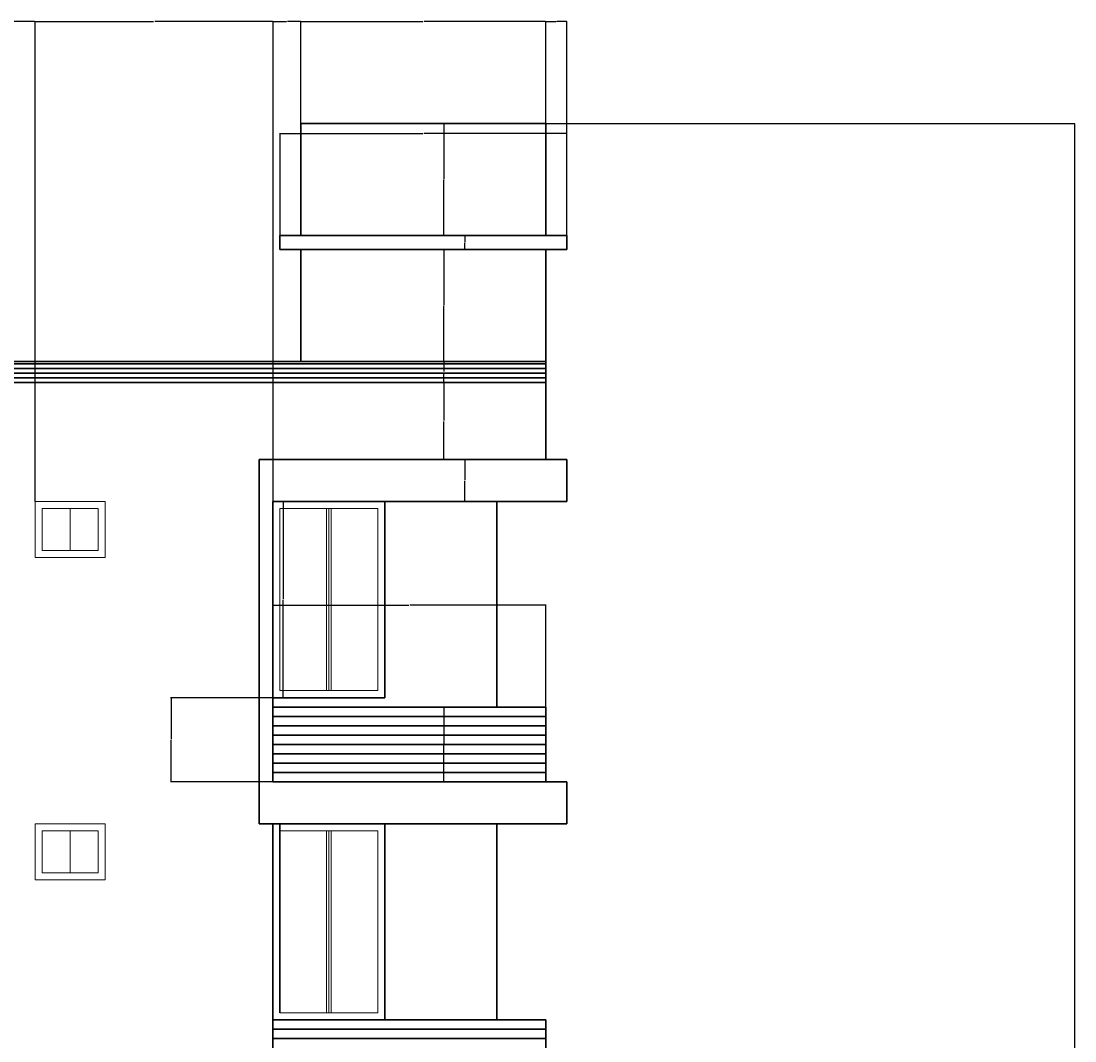
# Model space of a CAD drawing. Units: inches. Extents: x 2136 to 3058, y 322 to 1274.
# Tile 3 of 3: x 2606 to 3058, y 837 to 1274. Entities that reach past the tile are written whole.
import ezdxf

# ---------------------------------------------------------------- set-up
doc = ezdxf.new("R2010")
doc.units = ezdxf.units.IN
for name, color, linetype, lineweight in [('A-ANNO-DIMS', 2, 'Continuous', 18), ('A-ELEV', 7, 'Continuous', 35), ('A-GLAZ', 4, 'Continuous', 18)]:
    doc.layers.add(name, color=color, linetype=linetype, lineweight=lineweight)
doc.styles.get("Standard").update_dxf_attribs({"font": 'arial.ttf'})
doc.dimstyles.get("Standard").update_dxf_attribs({"dimtxt": 0.18, "dimasz": 0.18, "dimexe": 0.18, "dimexo": 0.0625, "dimgap": 0.09, "dimtad": 0, "dimtih": 1, "dimtoh": 1, "dimdec": 4, "dimzin": 0, "dimdsep": 46, "dimtxsty": 'Standard', "dimcen": 0.09, "dimadec": 0, "dimazin": 0, "dimtfac": 1, "dimtdec": 4, "dimtofl": 0, "dimtmove": 0, "dimatfit": 3, "dimfxl": 1, "dimtolj": 1, "dimtzin": 0, "dimarcsym": 0})

# ---------------------------------------------------------------- blocks, each defined once
blk = doc.blocks.new('WIN-SMALL')
for p, q in [((2458.76, 1064.68), (2434.76, 1064.68)), ((2434.76, 1064.68), (2434.76, 1046.68)), ((2446.76, 1064.68), (2446.76, 1046.68)), ((2458.76, 1064.68), (2458.76, 1046.68)), ((2458.76, 1046.68), (2434.76, 1046.68))]:
    blk.add_line(p, q)
blk = doc.blocks.new('WIN-TALL')
for p, q in [((2716.76, 650.68), (2716.76, 572.68)), ((2716.76, 650.68), (2758.76, 650.68)), ((2736.76, 650.68), (2736.76, 572.68)), ((2737.76, 650.68), (2737.76, 572.68)), ((2738.76, 650.68), (2738.76, 572.68)), ((2758.76, 650.68), (2758.76, 572.68)), ((2716.76, 572.68), (2758.76, 572.68))]:
    blk.add_line(p, q)
blk = doc.blocks.new('*D12')
at = {"layer": 'A-ANNO-DIMS', "color": 0, "lineweight": -2, "transparency": 16777216}
for p, q in [((2830.82, 1229.68), (3057.52, 1229.68)), ((3057.34, 1229.5), (3057.34, 797.87)), ((3057.34, 365.86), (3057.34, 797.5)), ((2839.82, 365.68), (3057.52, 365.68))]:
    blk.add_line(p, q, dxfattribs=at)
at = {"layer": 'A-ANNO-DIMS', "color": 0, "transparency": 16777216}
for points in [[(3057.31, 1229.5), (3057.37, 1229.5), (3057.34, 1229.68)], [(3057.31, 365.86), (3057.37, 365.86), (3057.34, 365.68)]]:
    blk.add_solid(points, dxfattribs=at)
at = {"layer": 'Defpoints', "color": 0, "transparency": 16777216}
for p in [(2830.76, 1229.68), (3057.34, 1229.68), (2839.76, 365.68)]:
    blk.add_point(p, dxfattribs=at)
at = {"layer": 'A-ANNO-DIMS', "color": 0, "transparency": 16777216, "insert": (3057.34, 797.68), "char_height": 0.18, "attachment_point": 5}
blk.add_mtext('\\A1;864', dxfattribs=at)
blk = doc.blocks.new('*D25')
at = {"layer": 'A-ANNO-DIMS', "color": 0, "lineweight": -2, "transparency": 16777216}
for p, q in [((2515.76, 1067.75), (2515.76, 1273.56)), ((2515.94, 1273.38), (2563.54, 1273.38)), ((2611.58, 1273.38), (2563.98, 1273.38)), ((2611.76, 1067.75), (2611.76, 1273.56))]:
    blk.add_line(p, q, dxfattribs=at)
at = {"layer": 'A-ANNO-DIMS', "color": 0, "transparency": 16777216}
for points in [[(2515.94, 1273.41), (2515.94, 1273.35), (2515.76, 1273.38)], [(2611.58, 1273.41), (2611.58, 1273.35), (2611.76, 1273.38)]]:
    blk.add_solid(points, dxfattribs=at)
at = {"layer": 'Defpoints', "color": 0, "transparency": 16777216}
for p in [(2611.76, 1273.38), (2515.76, 1067.68), (2611.76, 1067.68)]:
    blk.add_point(p, dxfattribs=at)
at = {"layer": 'A-ANNO-DIMS', "color": 0, "transparency": 16777216, "insert": (2563.76, 1273.38), "char_height": 0.18, "attachment_point": 5}
blk.add_mtext('\\A1;96', dxfattribs=at)
blk = doc.blocks.new('*D26')
at = {"layer": 'A-ANNO-DIMS', "color": 0, "lineweight": -2, "transparency": 16777216}
for p, q in [((2611.76, 1067.75), (2611.76, 1273.56)), ((2611.94, 1273.38), (2662.48, 1273.38)), ((2713.58, 1273.38), (2663.04, 1273.38)), ((2713.76, 1067.75), (2713.76, 1273.56))]:
    blk.add_line(p, q, dxfattribs=at)
at = {"layer": 'A-ANNO-DIMS', "color": 0, "transparency": 16777216}
for points in [[(2611.94, 1273.41), (2611.94, 1273.35), (2611.76, 1273.38)], [(2713.58, 1273.41), (2713.58, 1273.35), (2713.76, 1273.38)]]:
    blk.add_solid(points, dxfattribs=at)
at = {"layer": 'Defpoints', "color": 0, "transparency": 16777216}
for p in [(2713.76, 1273.38), (2611.76, 1067.68), (2713.76, 1067.68)]:
    blk.add_point(p, dxfattribs=at)
at = {"layer": 'A-ANNO-DIMS', "color": 0, "transparency": 16777216, "insert": (2662.76, 1273.38), "char_height": 0.18, "attachment_point": 5}
blk.add_mtext('\\A1;102', dxfattribs=at)
blk = doc.blocks.new('*D27')
at = {"layer": 'A-ANNO-DIMS', "color": 0, "lineweight": -2, "transparency": 16777216}
for p, q in [((2713.76, 1067.75), (2713.76, 1273.56)), ((2713.94, 1273.38), (2719.55, 1273.38)), ((2725.58, 1273.38), (2719.97, 1273.38)), ((2725.76, 1229.75), (2725.76, 1273.56))]:
    blk.add_line(p, q, dxfattribs=at)
at = {"layer": 'A-ANNO-DIMS', "color": 0, "transparency": 16777216}
for points in [[(2713.94, 1273.41), (2713.94, 1273.35), (2713.76, 1273.38)], [(2725.58, 1273.41), (2725.58, 1273.35), (2725.76, 1273.38)]]:
    blk.add_solid(points, dxfattribs=at)
at = {"layer": 'Defpoints', "color": 0, "transparency": 16777216}
for p in [(2725.76, 1273.38), (2725.76, 1229.68), (2713.76, 1067.68)]:
    blk.add_point(p, dxfattribs=at)
at = {"layer": 'A-ANNO-DIMS', "color": 0, "transparency": 16777216, "insert": (2719.76, 1273.38), "char_height": 0.18, "attachment_point": 5}
blk.add_mtext('\\A1;12', dxfattribs=at)
blk = doc.blocks.new('*D28')
at = {"layer": 'A-ANNO-DIMS', "color": 0, "lineweight": -2, "transparency": 16777216}
for p, q in [((2725.76, 1229.75), (2725.76, 1273.56)), ((2725.94, 1273.38), (2777.98, 1273.38)), ((2830.58, 1273.38), (2778.54, 1273.38)), ((2830.76, 1229.75), (2830.76, 1273.56))]:
    blk.add_line(p, q, dxfattribs=at)
at = {"layer": 'A-ANNO-DIMS', "color": 0, "transparency": 16777216}
for points in [[(2725.94, 1273.41), (2725.94, 1273.35), (2725.76, 1273.38)], [(2830.58, 1273.41), (2830.58, 1273.35), (2830.76, 1273.38)]]:
    blk.add_solid(points, dxfattribs=at)
at = {"layer": 'Defpoints', "color": 0, "transparency": 16777216}
for p in [(2830.76, 1273.38), (2725.76, 1229.68), (2830.76, 1229.68)]:
    blk.add_point(p, dxfattribs=at)
at = {"layer": 'A-ANNO-DIMS', "color": 0, "transparency": 16777216, "insert": (2778.26, 1273.38), "char_height": 0.18, "attachment_point": 5}
blk.add_mtext('\\A1;105', dxfattribs=at)
blk = doc.blocks.new('*D29')
at = {"layer": 'A-ANNO-DIMS', "color": 0, "lineweight": -2, "transparency": 16777216}
for p, q in [((2830.76, 1229.75), (2830.76, 1273.56)), ((2830.94, 1273.38), (2835.11, 1273.38)), ((2839.58, 1273.38), (2835.41, 1273.38)), ((2839.76, 1181.75), (2839.76, 1273.56))]:
    blk.add_line(p, q, dxfattribs=at)
at = {"layer": 'A-ANNO-DIMS', "color": 0, "transparency": 16777216}
for points in [[(2830.94, 1273.41), (2830.94, 1273.35), (2830.76, 1273.38)], [(2839.58, 1273.41), (2839.58, 1273.35), (2839.76, 1273.38)]]:
    blk.add_solid(points, dxfattribs=at)
at = {"layer": 'Defpoints', "color": 0, "transparency": 16777216}
for p in [(2839.76, 1273.38), (2830.76, 1229.68), (2839.76, 1181.68)]:
    blk.add_point(p, dxfattribs=at)
at = {"layer": 'A-ANNO-DIMS', "color": 0, "transparency": 16777216, "insert": (2835.26, 1273.38), "char_height": 0.18, "attachment_point": 5}
blk.add_mtext('\\A1;9', dxfattribs=at)
blk = doc.blocks.new('*D30')
at = {"layer": 'A-ANNO-DIMS', "color": 0, "lineweight": -2, "transparency": 16777216}
for p, q in [((2830.7, 1229.68), (2786.88, 1229.68)), ((2787.06, 1229.5), (2787.06, 1205.87)), ((2787.06, 1181.86), (2787.06, 1205.5)), ((2830.7, 1181.68), (2786.88, 1181.68))]:
    blk.add_line(p, q, dxfattribs=at)
at = {"layer": 'A-ANNO-DIMS', "color": 0, "transparency": 16777216}
for points in [[(2787.03, 1229.5), (2787.09, 1229.5), (2787.06, 1229.68)], [(2787.03, 1181.86), (2787.09, 1181.86), (2787.06, 1181.68)]]:
    blk.add_solid(points, dxfattribs=at)
at = {"layer": 'Defpoints', "color": 0, "transparency": 16777216}
for p in [(2787.06, 1229.68), (2830.76, 1229.68), (2830.76, 1181.68)]:
    blk.add_point(p, dxfattribs=at)
at = {"layer": 'A-ANNO-DIMS', "color": 0, "transparency": 16777216, "insert": (2787.06, 1205.68), "char_height": 0.18, "attachment_point": 5}
blk.add_mtext('\\A1;48', dxfattribs=at)
blk = doc.blocks.new('*D31')
at = {"layer": 'A-ANNO-DIMS', "color": 0, "lineweight": -2, "transparency": 16777216}
for p, q in [((2839.7, 1181.68), (2795.88, 1181.68)), ((2796.06, 1181.5), (2796.06, 1178.87)), ((2839.7, 1175.68), (2795.88, 1175.68)), ((2796.06, 1175.86), (2796.06, 1178.5))]:
    blk.add_line(p, q, dxfattribs=at)
at = {"layer": 'A-ANNO-DIMS', "color": 0, "transparency": 16777216}
for points in [[(2796.03, 1181.5), (2796.09, 1181.5), (2796.06, 1181.68)], [(2796.03, 1175.86), (2796.09, 1175.86), (2796.06, 1175.68)]]:
    blk.add_solid(points, dxfattribs=at)
at = {"layer": 'Defpoints', "color": 0, "transparency": 16777216}
for p in [(2796.06, 1181.68), (2839.76, 1181.68), (2839.76, 1175.68)]:
    blk.add_point(p, dxfattribs=at)
at = {"layer": 'A-ANNO-DIMS', "color": 0, "transparency": 16777216, "insert": (2796.06, 1178.68), "char_height": 0.18, "attachment_point": 5}
blk.add_mtext('\\A1;6', dxfattribs=at)
blk = doc.blocks.new('*D32')
at = {"layer": 'A-ANNO-DIMS', "color": 0, "lineweight": -2, "transparency": 16777216}
for p, q in [((2830.7, 1175.68), (2786.88, 1175.68)), ((2787.06, 1175.5), (2787.06, 1151.87)), ((2787.06, 1127.86), (2787.06, 1151.5)), ((2830.7, 1127.68), (2786.88, 1127.68))]:
    blk.add_line(p, q, dxfattribs=at)
at = {"layer": 'A-ANNO-DIMS', "color": 0, "transparency": 16777216}
for points in [[(2787.03, 1175.5), (2787.09, 1175.5), (2787.06, 1175.68)], [(2787.03, 1127.86), (2787.09, 1127.86), (2787.06, 1127.68)]]:
    blk.add_solid(points, dxfattribs=at)
at = {"layer": 'Defpoints', "color": 0, "transparency": 16777216}
for p in [(2787.06, 1175.68), (2830.76, 1175.68), (2830.76, 1127.68)]:
    blk.add_point(p, dxfattribs=at)
at = {"layer": 'A-ANNO-DIMS', "color": 0, "transparency": 16777216, "insert": (2787.06, 1151.68), "char_height": 0.18, "attachment_point": 5}
blk.add_mtext('\\A1;48', dxfattribs=at)
blk = doc.blocks.new('*D33')
at = {"layer": 'A-ANNO-DIMS', "color": 0, "lineweight": -2, "transparency": 16777216}
for p, q in [((2830.7, 1127.68), (2786.88, 1127.68)), ((2787.06, 1127.5), (2787.06, 1123.37)), ((2787.06, 1118.86), (2787.06, 1123)), ((2830.7, 1118.68), (2786.88, 1118.68))]:
    blk.add_line(p, q, dxfattribs=at)
at = {"layer": 'A-ANNO-DIMS', "color": 0, "transparency": 16777216}
for points in [[(2787.03, 1127.5), (2787.09, 1127.5), (2787.06, 1127.68)], [(2787.03, 1118.86), (2787.09, 1118.86), (2787.06, 1118.68)]]:
    blk.add_solid(points, dxfattribs=at)
at = {"layer": 'Defpoints', "color": 0, "transparency": 16777216}
for p in [(2787.06, 1127.68), (2830.76, 1127.68), (2830.76, 1118.68)]:
    blk.add_point(p, dxfattribs=at)
at = {"layer": 'A-ANNO-DIMS', "color": 0, "transparency": 16777216, "insert": (2787.06, 1123.18), "char_height": 0.18, "attachment_point": 5}
blk.add_mtext('\\A1;9', dxfattribs=at)
blk = doc.blocks.new('*D34')
at = {"layer": 'A-ANNO-DIMS', "color": 0, "lineweight": -2, "transparency": 16777216}
for p, q in [((2830.7, 1118.68), (2786.88, 1118.68)), ((2787.06, 1118.5), (2787.06, 1102.37)), ((2787.06, 1085.86), (2787.06, 1102)), ((2830.7, 1085.68), (2786.88, 1085.68))]:
    blk.add_line(p, q, dxfattribs=at)
at = {"layer": 'A-ANNO-DIMS', "color": 0, "transparency": 16777216}
for points in [[(2787.03, 1118.5), (2787.09, 1118.5), (2787.06, 1118.68)], [(2787.03, 1085.86), (2787.09, 1085.86), (2787.06, 1085.68)]]:
    blk.add_solid(points, dxfattribs=at)
at = {"layer": 'Defpoints', "color": 0, "transparency": 16777216}
for p in [(2787.06, 1118.68), (2830.76, 1118.68), (2830.76, 1085.68)]:
    blk.add_point(p, dxfattribs=at)
at = {"layer": 'A-ANNO-DIMS', "color": 0, "transparency": 16777216, "insert": (2787.06, 1102.18), "char_height": 0.18, "attachment_point": 5}
blk.add_mtext('\\A1;33', dxfattribs=at)
blk = doc.blocks.new('*D35')
at = {"layer": 'A-ANNO-DIMS', "color": 0, "lineweight": -2, "transparency": 16777216}
for p, q in [((2839.7, 1085.68), (2795.88, 1085.68)), ((2796.06, 1085.5), (2796.06, 1076.87)), ((2796.06, 1067.86), (2796.06, 1076.5)), ((2839.7, 1067.68), (2795.88, 1067.68))]:
    blk.add_line(p, q, dxfattribs=at)
at = {"layer": 'A-ANNO-DIMS', "color": 0, "transparency": 16777216}
for points in [[(2796.03, 1085.5), (2796.09, 1085.5), (2796.06, 1085.68)], [(2796.03, 1067.86), (2796.09, 1067.86), (2796.06, 1067.68)]]:
    blk.add_solid(points, dxfattribs=at)
at = {"layer": 'Defpoints', "color": 0, "transparency": 16777216}
for p in [(2796.06, 1085.68), (2839.76, 1085.68), (2839.76, 1067.68)]:
    blk.add_point(p, dxfattribs=at)
at = {"layer": 'A-ANNO-DIMS', "color": 0, "transparency": 16777216, "insert": (2796.06, 1076.68), "char_height": 0.18, "attachment_point": 5}
blk.add_mtext('\\A1;18', dxfattribs=at)
blk = doc.blocks.new('*D36')
at = {"layer": 'A-ANNO-DIMS', "color": 0, "lineweight": -2, "transparency": 16777216}
for p, q in [((2761.7, 1067.68), (2717.88, 1067.68)), ((2718.06, 1067.5), (2718.06, 1025.87)), ((2718.06, 983.86), (2718.06, 1025.5)), ((2761.7, 983.68), (2717.88, 983.68))]:
    blk.add_line(p, q, dxfattribs=at)
at = {"layer": 'A-ANNO-DIMS', "color": 0, "transparency": 16777216}
for points in [[(2718.03, 1067.5), (2718.09, 1067.5), (2718.06, 1067.68)], [(2718.03, 983.86), (2718.09, 983.86), (2718.06, 983.68)]]:
    blk.add_solid(points, dxfattribs=at)
at = {"layer": 'Defpoints', "color": 0, "transparency": 16777216}
for p in [(2718.06, 1067.68), (2761.76, 1067.68), (2761.76, 983.68)]:
    blk.add_point(p, dxfattribs=at)
at = {"layer": 'A-ANNO-DIMS', "color": 0, "transparency": 16777216, "insert": (2718.06, 1025.68), "char_height": 0.18, "attachment_point": 5}
blk.add_mtext('\\A1;84', dxfattribs=at)
blk = doc.blocks.new('*D37')
at = {"layer": 'A-ANNO-DIMS', "color": 0, "lineweight": -2, "transparency": 16777216}
for p, q in [((2713.7, 983.68), (2669.88, 983.68)), ((2670.06, 983.5), (2670.06, 965.87)), ((2670.06, 947.86), (2670.06, 965.5)), ((2713.7, 947.68), (2669.88, 947.68))]:
    blk.add_line(p, q, dxfattribs=at)
at = {"layer": 'A-ANNO-DIMS', "color": 0, "transparency": 16777216}
for points in [[(2670.03, 983.5), (2670.09, 983.5), (2670.06, 983.68)], [(2670.03, 947.86), (2670.09, 947.86), (2670.06, 947.68)]]:
    blk.add_solid(points, dxfattribs=at)
at = {"layer": 'Defpoints', "color": 0, "transparency": 16777216}
for p in [(2670.06, 983.68), (2713.76, 983.68), (2713.76, 947.68)]:
    blk.add_point(p, dxfattribs=at)
at = {"layer": 'A-ANNO-DIMS', "color": 0, "transparency": 16777216, "insert": (2670.06, 965.68), "char_height": 0.18, "attachment_point": 5}
blk.add_mtext('\\A1;36', dxfattribs=at)
blk = doc.blocks.new('*D38')
at = {"layer": 'A-ANNO-DIMS', "color": 0, "lineweight": -2, "transparency": 16777216}
for p, q in [((2830.7, 979.68), (2786.88, 979.68)), ((2787.06, 979.5), (2787.06, 963.87)), ((2787.06, 947.86), (2787.06, 963.5)), ((2830.7, 947.68), (2786.88, 947.68))]:
    blk.add_line(p, q, dxfattribs=at)
at = {"layer": 'A-ANNO-DIMS', "color": 0, "transparency": 16777216}
for points in [[(2787.03, 979.5), (2787.09, 979.5), (2787.06, 979.68)], [(2787.03, 947.86), (2787.09, 947.86), (2787.06, 947.68)]]:
    blk.add_solid(points, dxfattribs=at)
at = {"layer": 'Defpoints', "color": 0, "transparency": 16777216}
for p in [(2787.06, 979.68), (2830.76, 979.68), (2830.76, 947.68)]:
    blk.add_point(p, dxfattribs=at)
at = {"layer": 'A-ANNO-DIMS', "color": 0, "transparency": 16777216, "insert": (2787.06, 963.68), "char_height": 0.18, "attachment_point": 5}
blk.add_mtext('\\A1;32', dxfattribs=at)
blk = doc.blocks.new('*D40')
at = {"layer": 'A-ANNO-DIMS', "color": 0, "lineweight": -2, "transparency": 16777216}
for p, q in [((2716.76, 1181.75), (2716.76, 1225.56)), ((2716.94, 1225.38), (2777.98, 1225.38)), ((2839.58, 1225.38), (2778.54, 1225.38)), ((2839.76, 1181.75), (2839.76, 1225.56))]:
    blk.add_line(p, q, dxfattribs=at)
at = {"layer": 'A-ANNO-DIMS', "color": 0, "transparency": 16777216}
for points in [[(2716.94, 1225.41), (2716.94, 1225.35), (2716.76, 1225.38)], [(2839.58, 1225.41), (2839.58, 1225.35), (2839.76, 1225.38)]]:
    blk.add_solid(points, dxfattribs=at)
at = {"layer": 'Defpoints', "color": 0, "transparency": 16777216}
for p in [(2839.76, 1225.38), (2716.76, 1181.68), (2839.76, 1181.68)]:
    blk.add_point(p, dxfattribs=at)
at = {"layer": 'A-ANNO-DIMS', "color": 0, "transparency": 16777216, "insert": (2778.26, 1225.38), "char_height": 0.18, "attachment_point": 5}
blk.add_mtext('\\A1;123', dxfattribs=at)
blk = doc.blocks.new('*D42')
at = {"layer": 'A-ANNO-DIMS', "color": 0, "lineweight": -2, "transparency": 16777216}
for p, q in [((2713.76, 979.75), (2713.76, 1023.56)), ((2713.94, 1023.38), (2771.98, 1023.38)), ((2830.58, 1023.38), (2772.54, 1023.38)), ((2830.76, 979.75), (2830.76, 1023.56))]:
    blk.add_line(p, q, dxfattribs=at)
at = {"layer": 'A-ANNO-DIMS', "color": 0, "transparency": 16777216}
for points in [[(2713.94, 1023.41), (2713.94, 1023.35), (2713.76, 1023.38)], [(2830.58, 1023.41), (2830.58, 1023.35), (2830.76, 1023.38)]]:
    blk.add_solid(points, dxfattribs=at)
at = {"layer": 'Defpoints', "color": 0, "transparency": 16777216}
for p in [(2830.76, 1023.38), (2713.76, 979.68), (2830.76, 979.68)]:
    blk.add_point(p, dxfattribs=at)
at = {"layer": 'A-ANNO-DIMS', "color": 0, "transparency": 16777216, "insert": (2772.26, 1023.38), "char_height": 0.18, "attachment_point": 5}
blk.add_mtext('\\A1;117', dxfattribs=at)

msp = doc.modelspace()

# ---------------------------------------------------------------- linework, layer by layer
at = {"layer": 'A-ELEV'}
for p, q in [((2725.759, 1229.684), (2725.759, 1181.684)), ((2725.759, 1229.684), (2830.759, 1229.684)), ((2830.759, 1229.684), (2830.759, 1181.684)), ((2716.759, 1181.684), (2839.759, 1181.684)), ((2716.759, 1181.684), (2716.759, 1175.684)), ((2839.759, 1181.684), (2839.759, 1175.684)), ((2716.759, 1175.684), (2839.759, 1175.684)), ((2725.759, 1175.684), (2725.759, 1127.684)), ((2830.759, 1175.684), (2830.759, 1085.684)), ((2194.759, 1127.684), (2830.759, 1127.684)), ((2419.759, 1126.684), (2830.759, 1126.684)), ((2419.759, 1124.684), (2830.759, 1124.684)), ((2419.759, 1122.684), (2830.759, 1122.684)), ((2419.759, 1120.684), (2830.759, 1120.684)), ((2419.759, 1118.684), (2830.759, 1118.684)), ((2707.759, 1085.684), (2839.759, 1085.684)), ((2707.759, 1085.684), (2707.759, 929.684)), ((2839.759, 1085.684), (2839.759, 1067.684)), ((2713.759, 1067.684), (2713.759, 947.684)), ((2713.759, 1067.684), (2839.759, 1067.684)), ((2761.759, 1067.684), (2761.759, 983.684)), ((2809.759, 1067.684), (2809.759, 979.684)), ((2713.759, 983.684), (2761.759, 983.684)), ((2713.759, 979.684), (2830.759, 979.684)), ((2830.759, 979.684), (2830.759, 947.684)), ((2713.759, 975.684), (2830.759, 975.684)), ((2713.759, 971.684), (2830.759, 971.684)), ((2713.759, 967.684), (2830.759, 967.684)), ((2713.759, 963.684), (2830.759, 963.684)), ((2713.759, 959.684), (2830.759, 959.684)), ((2713.759, 955.684), (2830.759, 955.684)), ((2713.759, 951.684), (2830.759, 951.684)), ((2713.759, 947.684), (2839.759, 947.684)), ((2839.759, 947.684), (2839.759, 929.684)), ((2707.759, 929.684), (2839.759, 929.684)), ((2713.759, 929.684), (2713.759, 841.684)), ((2716.759, 929.684), (2716.759, 848.684)), ((2761.759, 929.684), (2761.759, 845.684)), ((2809.759, 929.684), (2809.759, 845.684)), ((2713.759, 845.684), (2830.759, 845.684)), ((2713.759, 845.684), (2761.759, 845.684)), ((2830.759, 809.684), (2830.759, 845.684)), ((2713.759, 841.684), (2830.759, 841.684)), ((2713.759, 841.684), (2713.759, 809.684)), ((2713.759, 837.684), (2830.759, 837.684))]:
    msp.add_line(p, q, dxfattribs=at)
at = {"layer": 'A-GLAZ'}
for p, q in [((2641.759, 1067.684), (2611.759, 1067.684)), ((2611.759, 1067.684), (2611.759, 1043.684)), ((2641.759, 1067.684), (2641.759, 1043.684)), ((2641.759, 1043.684), (2611.759, 1043.684)), ((2641.759, 929.684), (2611.759, 929.684)), ((2611.759, 929.684), (2611.759, 905.684)), ((2641.759, 929.684), (2641.759, 905.684)), ((2716.759, 926.684), (2758.759, 926.684)), ((2736.759, 926.684), (2736.759, 848.684)), ((2737.759, 926.684), (2737.759, 848.684)), ((2738.759, 926.684), (2738.759, 848.684)), ((2758.759, 926.684), (2758.759, 848.684)), ((2641.759, 905.684), (2611.759, 905.684)), ((2716.759, 848.684), (2758.759, 848.684))]:
    msp.add_line(p, q, dxfattribs=at)

# ---------------------------------------------------------------- block references
for p in [(180, 0), (180, -138)]:
    msp.add_blockref('WIN-SMALL', p, dxfattribs=at)
at = {"layer": 'A-GLAZ', "rotation": 180}
msp.add_blockref('WIN-TALL', (5475.519, 1637.367), dxfattribs=at)

# ---------------------------------------------------------------- dimensions: what is measured, and where the dimension line sits
at = {"layer": 'A-ANNO-DIMS'}
for base, p1, p2, picture, middle in [((2611.759, 1273.384), (2515.759, 1067.684), (2611.759, 1067.684), '*D25', (2563.759, 1273.384)), ((2713.759, 1273.384), (2611.759, 1067.684), (2713.759, 1067.684), '*D26', (2662.759, 1273.384)), ((2725.759, 1273.384), (2713.759, 1067.684), (2725.759, 1229.684), '*D27', (2719.759, 1273.384)), ((2830.759, 1273.384), (2725.759, 1229.684), (2830.759, 1229.684), '*D28', (2778.259, 1273.384)), ((2839.759, 1273.384), (2830.759, 1229.684), (2839.759, 1181.684), '*D29', (2835.259, 1273.384)), ((2839.759, 1225.384), (2716.759, 1181.684), (2839.759, 1181.684), '*D40', (2778.259, 1225.384)), ((2830.759, 1023.384), (2713.759, 979.684), (2830.759, 979.684), '*D42', (2772.259, 1023.384))]:
    dim = msp.add_linear_dim(base=base, p1=p1, p2=p2, dimstyle='Standard', override={"dimdec": 0, "dimlfac": 1, "dimrnd": 0, "dimzin": 0, "dimdsep": 46, "dimlunit": 2}, dxfattribs=at)
    dim.commit()
    dim.dimension.update_dxf_attribs({"geometry": picture, "text_midpoint": middle})
for base, p1, p2, picture, middle in [((2787.059, 1229.684), (2830.759, 1181.684), (2830.759, 1229.684), '*D30', (2787.059, 1205.684)), ((3057.34, 1229.684), (2839.759, 365.684), (2830.759, 1229.684), '*D12', (3057.34, 797.684)), ((2796.059, 1181.684), (2839.759, 1175.684), (2839.759, 1181.684), '*D31', (2796.059, 1178.684)), ((2787.059, 1175.684), (2830.759, 1127.684), (2830.759, 1175.684), '*D32', (2787.059, 1151.684)), ((2787.059, 1127.684), (2830.759, 1118.684), (2830.759, 1127.684), '*D33', (2787.059, 1123.184)), ((2787.059, 1118.684), (2830.759, 1085.684), (2830.759, 1118.684), '*D34', (2787.059, 1102.184)), ((2796.059, 1085.684), (2839.759, 1067.684), (2839.759, 1085.684), '*D35', (2796.059, 1076.684)), ((2718.059, 1067.684), (2761.759, 983.684), (2761.759, 1067.684), '*D36', (2718.059, 1025.684)), ((2670.059, 983.684), (2713.759, 947.684), (2713.759, 983.684), '*D37', (2670.059, 965.684)), ((2787.059, 979.684), (2830.759, 947.684), (2830.759, 979.684), '*D38', (2787.059, 963.684))]:
    dim = msp.add_linear_dim(base=base, p1=p1, p2=p2, angle=90, dimstyle='Standard', override={"dimdec": 0, "dimlfac": 1, "dimrnd": 0, "dimzin": 0, "dimdsep": 46, "dimlunit": 2}, dxfattribs=at)
    dim.commit()
    dim.dimension.update_dxf_attribs({"geometry": picture, "text_midpoint": middle})

doc.saveas('drawing.dxf')
